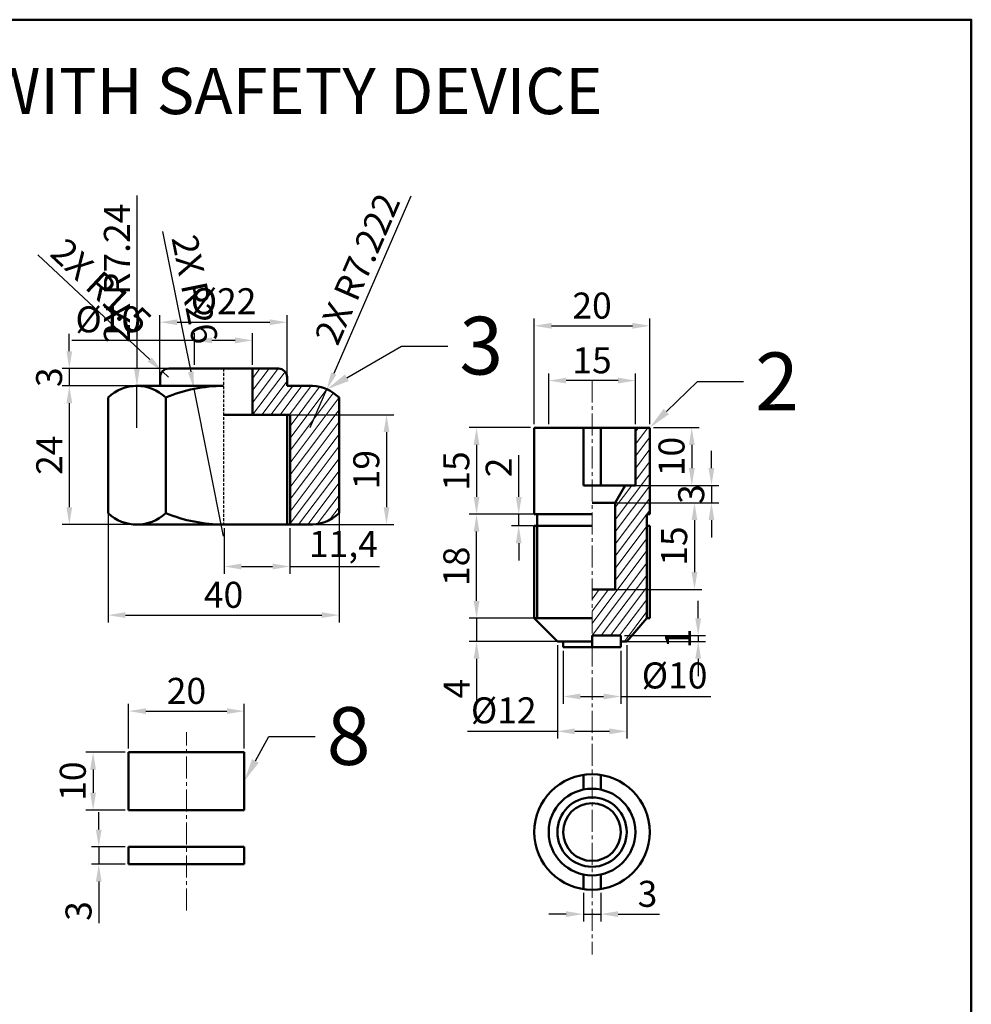
# Model space of a CAD drawing. Units: millimetres. Extents: x 418 to 773, y -46 to 294.
# Tile 7 of 7: x 609 to 773, y 124 to 294. Entities that reach past the tile are written whole.
import ezdxf
from ezdxf import colors
from ezdxf.entities.mleader import LeaderData, LeaderLine
from ezdxf.math import Vec2, Vec3

# ---------------------------------------------------------------- set-up
doc = ezdxf.new("R2010")
doc.units = ezdxf.units.MM
doc.header["$LTSCALE"] = 0.2
doc.linetypes.add('CENTER2', pattern=[28.575, 19.05, -3.175, 3.175, -3.175])
doc.linetypes.add('DASHED', pattern=[19.05, 12.7, -6.35])
for name, color, linetype, lineweight in [('M-CNTR', 1, 'CENTER2', 18), ('M-DIMS', 2, 'Continuous', 25), ('M-HATC', 8, 'Continuous', 18), ('M-HIDN', 4, 'DASHED', 25), ('M-OUTL', 7, 'Continuous', 50), ('M-TEXT', 3, 'Continuous', 25), ('M-TTLB', 7, 'Continuous', 50)]:
    doc.layers.add(name, color=color, linetype=linetype, lineweight=lineweight)
doc.styles.get("Standard").update_dxf_attribs({"font": 'arial.ttf'})
doc.dimstyles.new('ISO-25', dxfattribs={"dimtxt": 4.5, "dimasz": 3, "dimexe": 1.25, "dimexo": 0.625, "dimtad": 1, "dimdec": 1, "dimtxsty": 'Standard', "dimcen": 2.5, "dimadec": 0, "dimazin": 0, "dimtfac": 1, "dimtdec": 1, "dimtmove": 0, "dimatfit": 3, "dimfxl": 1, "dimarcsym": 0})

# ---------------------------------------------------------------- blocks, each defined once
blk = doc.blocks.new('*D43')
at = {"layer": 'Defpoints', "color": 0, "ltscale": 0.2, "transparency": 16777216}
for p in [(643.92, 207.02), (655.34, 207.02), (655.34, 199.76)]:
    blk.add_point(p, dxfattribs=at)
at = {"layer": 'M-DIMS', "color": 0, "lineweight": -2, "ltscale": 0.2, "transparency": 16777216}
for p, q in [((643.92, 206.39), (643.92, 198.51)), ((655.34, 206.39), (655.34, 198.51)), ((646.92, 199.76), (652.34, 199.76)), ((655.34, 199.76), (670.84, 199.76))]:
    blk.add_line(p, q, dxfattribs=at)
at = {"layer": 'M-DIMS', "color": 0, "ltscale": 0.2, "transparency": 16777216}
for points in [[(646.92, 200.26), (646.92, 199.26), (643.92, 199.76)], [(652.34, 200.26), (652.34, 199.26), (655.34, 199.76)]]:
    blk.add_solid(points, dxfattribs=at)
at = {"layer": 'M-DIMS', "color": 0, "ltscale": 0.2, "transparency": 16777216, "insert": (664.59, 203.09), "char_height": 4.5, "attachment_point": 5}
blk.add_mtext('11,4', dxfattribs=at)
blk = doc.blocks.new('*D44')
at = {"layer": 'Defpoints', "color": 0, "ltscale": 0.2, "transparency": 16777216}
for p in [(623.84, 214.93), (663.84, 214.93), (663.84, 191.34)]:
    blk.add_point(p, dxfattribs=at)
at = {"layer": 'M-DIMS', "color": 0, "lineweight": -2, "ltscale": 0.2, "transparency": 16777216}
for p, q in [((623.84, 214.31), (623.84, 190.09)), ((663.84, 214.31), (663.84, 190.09)), ((626.84, 191.34), (660.84, 191.34))]:
    blk.add_line(p, q, dxfattribs=at)
at = {"layer": 'M-DIMS', "color": 0, "ltscale": 0.2, "transparency": 16777216}
for points in [[(626.84, 191.84), (626.84, 190.84), (623.84, 191.34)], [(660.84, 191.84), (660.84, 190.84), (663.84, 191.34)]]:
    blk.add_solid(points, dxfattribs=at)
at = {"layer": 'M-DIMS', "color": 0, "ltscale": 0.2, "transparency": 16777216, "insert": (643.84, 194.27), "char_height": 4.5, "attachment_point": 5}
blk.add_mtext('40', dxfattribs=at)
blk = doc.blocks.new('*D45')
at = {"layer": 'Defpoints', "color": 0, "ltscale": 0.2, "transparency": 16777216}
for p in [(654.84, 226.02), (654.84, 207.02), (672.05, 207.02)]:
    blk.add_point(p, dxfattribs=at)
at = {"layer": 'M-DIMS', "color": 0, "lineweight": -2, "ltscale": 0.2, "transparency": 16777216}
for p, q in [((655.47, 226.02), (673.3, 226.02)), ((672.05, 223.02), (672.05, 210.02)), ((655.47, 207.02), (673.3, 207.02))]:
    blk.add_line(p, q, dxfattribs=at)
at = {"layer": 'M-DIMS', "color": 0, "ltscale": 0.2, "transparency": 16777216}
for points in [[(671.55, 223.02), (672.55, 223.02), (672.05, 226.02)], [(671.55, 210.02), (672.55, 210.02), (672.05, 207.02)]]:
    blk.add_solid(points, dxfattribs=at)
at = {"layer": 'M-DIMS', "color": 0, "ltscale": 0.2, "transparency": 16777216, "insert": (669.13, 216.52), "char_height": 4.5, "attachment_point": 5, "rotation": 90}
blk.add_mtext('19', dxfattribs=at)
blk = doc.blocks.new('*D46')
at = {"layer": 'Defpoints', "color": 0, "ltscale": 0.2, "transparency": 16777216}
for p in [(632.84, 231.02), (617.14, 207.02), (632.84, 207.02)]:
    blk.add_point(p, dxfattribs=at)
at = {"layer": 'M-DIMS', "color": 0, "lineweight": -2, "ltscale": 0.2, "transparency": 16777216}
for p, q in [((632.22, 231.02), (615.89, 231.02)), ((617.14, 228.02), (617.14, 210.02)), ((632.22, 207.02), (615.89, 207.02))]:
    blk.add_line(p, q, dxfattribs=at)
at = {"layer": 'M-DIMS', "color": 0, "ltscale": 0.2, "transparency": 16777216}
for points in [[(616.64, 228.02), (617.64, 228.02), (617.14, 231.02)], [(616.64, 210.02), (617.64, 210.02), (617.14, 207.02)]]:
    blk.add_solid(points, dxfattribs=at)
at = {"layer": 'M-DIMS', "color": 0, "ltscale": 0.2, "transparency": 16777216, "insert": (614.26, 219.02), "char_height": 4.5, "attachment_point": 5, "rotation": 90}
blk.add_mtext('24', dxfattribs=at)
blk = doc.blocks.new('*D47')
at = {"layer": 'Defpoints', "color": 0, "ltscale": 0.2, "transparency": 16777216}
for p in [(642.2, 234.02), (617.14, 231.02), (642.2, 231.02)]:
    blk.add_point(p, dxfattribs=at)
at = {"layer": 'M-DIMS', "color": 0, "lineweight": -2, "ltscale": 0.2, "transparency": 16777216}
for p, q in [((617.14, 237.02), (617.14, 240.02)), ((641.58, 234.02), (615.89, 234.02)), ((617.14, 234.02), (617.14, 231.02)), ((641.58, 231.02), (615.89, 231.02)), ((617.14, 228.02), (617.14, 225.02))]:
    blk.add_line(p, q, dxfattribs=at)
at = {"layer": 'M-DIMS', "color": 0, "ltscale": 0.2, "transparency": 16777216}
for points in [[(616.64, 237.02), (617.64, 237.02), (617.14, 234.02)], [(616.64, 228.02), (617.64, 228.02), (617.14, 231.02)]]:
    blk.add_solid(points, dxfattribs=at)
at = {"layer": 'M-DIMS', "color": 0, "ltscale": 0.2, "transparency": 16777216, "insert": (614.22, 232.52), "char_height": 4.5, "attachment_point": 5, "rotation": 90}
blk.add_mtext('3', dxfattribs=at)
blk = doc.blocks.new('*D48')
at = {"layer": 'Defpoints', "color": 0, "ltscale": 0.2, "transparency": 16777216}
for p in [(654.84, 242.04), (632.84, 231.02), (654.84, 231.02)]:
    blk.add_point(p, dxfattribs=at)
at = {"layer": 'M-DIMS', "color": 0, "lineweight": -2, "ltscale": 0.2, "transparency": 16777216}
for p, q in [((632.84, 231.64), (632.84, 243.29)), ((635.84, 242.04), (651.84, 242.04)), ((654.84, 231.64), (654.84, 243.29))]:
    blk.add_line(p, q, dxfattribs=at)
at = {"layer": 'M-DIMS', "color": 0, "ltscale": 0.2, "transparency": 16777216}
for points in [[(635.84, 242.54), (635.84, 241.54), (632.84, 242.04)], [(651.84, 242.54), (651.84, 241.54), (654.84, 242.04)]]:
    blk.add_solid(points, dxfattribs=at)
at = {"layer": 'M-DIMS', "color": 0, "ltscale": 0.2, "transparency": 16777216, "insert": (643.84, 245.09), "char_height": 4.5, "attachment_point": 5}
blk.add_mtext('%%C22', dxfattribs=at)
blk = doc.blocks.new('*D49')
at = {"layer": 'Defpoints', "color": 0, "ltscale": 0.2, "transparency": 16777216}
for p in [(638.84, 238.9), (638.84, 234.02), (648.84, 234.02)]:
    blk.add_point(p, dxfattribs=at)
at = {"layer": 'M-DIMS', "color": 0, "lineweight": -2, "ltscale": 0.2, "transparency": 16777216}
for p, q in [((638.84, 238.9), (617.6, 238.9)), ((638.84, 234.64), (638.84, 240.15)), ((645.84, 238.9), (641.84, 238.9)), ((648.84, 234.64), (648.84, 240.15))]:
    blk.add_line(p, q, dxfattribs=at)
at = {"layer": 'M-DIMS', "color": 0, "ltscale": 0.2, "transparency": 16777216}
for points in [[(641.84, 239.4), (641.84, 238.4), (638.84, 238.9)], [(645.84, 239.4), (645.84, 238.4), (648.84, 238.9)]]:
    blk.add_solid(points, dxfattribs=at)
at = {"layer": 'M-DIMS', "color": 0, "ltscale": 0.2, "transparency": 16777216, "insert": (623.89, 241.95), "char_height": 4.5, "attachment_point": 5}
blk.add_mtext('%%C10', dxfattribs=at)
blk = doc.blocks.new('*U50')
at = {"layer": 'M-CNTR', "color": 0, "transparency": 16777216}
blk.add_line((0, -22.42), (0, 8.5), dxfattribs=at)
blk = doc.blocks.new('*D51')
at = {"layer": 'Defpoints', "color": 0, "ltscale": 0.2, "transparency": 16777216}
for p in [(647.41, 174.72), (627.41, 167.6), (647.41, 167.6)]:
    blk.add_point(p, dxfattribs=at)
at = {"layer": 'M-DIMS', "color": 0, "lineweight": -2, "ltscale": 0.2, "transparency": 16777216}
for p, q in [((627.41, 168.23), (627.41, 175.97)), ((647.41, 168.23), (647.41, 175.97)), ((630.41, 174.72), (644.41, 174.72))]:
    blk.add_line(p, q, dxfattribs=at)
at = {"layer": 'M-DIMS', "color": 0, "ltscale": 0.2, "transparency": 16777216}
for points in [[(630.41, 175.22), (630.41, 174.22), (627.41, 174.72)], [(644.41, 175.22), (644.41, 174.22), (647.41, 174.72)]]:
    blk.add_solid(points, dxfattribs=at)
at = {"layer": 'M-DIMS', "color": 0, "ltscale": 0.2, "transparency": 16777216, "insert": (637.41, 177.64), "char_height": 4.5, "attachment_point": 5}
blk.add_mtext('20', dxfattribs=at)
blk = doc.blocks.new('*D52')
at = {"layer": 'Defpoints', "color": 0, "ltscale": 0.2, "transparency": 16777216}
for p in [(627.41, 167.6), (621.26, 157.6), (627.41, 157.6)]:
    blk.add_point(p, dxfattribs=at)
at = {"layer": 'M-DIMS', "color": 0, "lineweight": -2, "ltscale": 0.2, "transparency": 16777216}
for p, q in [((626.79, 167.6), (620.01, 167.6)), ((621.26, 164.6), (621.26, 160.6)), ((626.79, 157.6), (620.01, 157.6))]:
    blk.add_line(p, q, dxfattribs=at)
at = {"layer": 'M-DIMS', "color": 0, "ltscale": 0.2, "transparency": 16777216}
for points in [[(620.76, 164.6), (621.76, 164.6), (621.26, 167.6)], [(620.76, 160.6), (621.76, 160.6), (621.26, 157.6)]]:
    blk.add_solid(points, dxfattribs=at)
at = {"layer": 'M-DIMS', "color": 0, "ltscale": 0.2, "transparency": 16777216, "insert": (618.33, 162.6), "char_height": 4.5, "attachment_point": 5, "rotation": 90}
blk.add_mtext('10', dxfattribs=at)
blk = doc.blocks.new('*D53')
at = {"layer": 'Defpoints', "color": 0, "ltscale": 0.2, "transparency": 16777216}
for p in [(627.41, 151.22), (622.24, 148.22), (627.41, 148.22)]:
    blk.add_point(p, dxfattribs=at)
at = {"layer": 'M-DIMS', "color": 0, "lineweight": -2, "ltscale": 0.2, "transparency": 16777216}
for p, q in [((622.24, 154.22), (622.24, 157.22)), ((626.79, 151.22), (620.99, 151.22)), ((622.24, 151.22), (622.24, 148.22)), ((626.79, 148.22), (620.99, 148.22)), ((622.24, 145.22), (622.24, 138.03))]:
    blk.add_line(p, q, dxfattribs=at)
at = {"layer": 'M-DIMS', "color": 0, "ltscale": 0.2, "transparency": 16777216}
for points in [[(621.74, 154.22), (622.74, 154.22), (622.24, 151.22)], [(621.74, 145.22), (622.74, 145.22), (622.24, 148.22)]]:
    blk.add_solid(points, dxfattribs=at)
at = {"layer": 'M-DIMS', "color": 0, "ltscale": 0.2, "transparency": 16777216, "insert": (619.32, 140.12), "char_height": 4.5, "attachment_point": 5, "rotation": 90}
blk.add_mtext('3', dxfattribs=at)
blk = doc.blocks.new('*U54')
at = {"layer": 'M-CNTR', "color": 0, "transparency": 16777216}
blk.add_line((0, 24.41), (0, -74.97), dxfattribs=at)
blk = doc.blocks.new('*D55')
at = {"layer": 'Defpoints', "color": 0, "ltscale": 0.2, "transparency": 16777216}
for p in [(717.62, 241.42), (697.62, 223.79), (717.62, 223.79)]:
    blk.add_point(p, dxfattribs=at)
at = {"layer": 'M-DIMS', "color": 0, "lineweight": -2, "ltscale": 0.2, "transparency": 16777216}
for p, q in [((697.62, 224.41), (697.62, 242.67)), ((717.62, 224.41), (717.62, 242.67)), ((700.62, 241.42), (714.62, 241.42))]:
    blk.add_line(p, q, dxfattribs=at)
at = {"layer": 'M-DIMS', "color": 0, "ltscale": 0.2, "transparency": 16777216}
for points in [[(700.62, 241.92), (700.62, 240.92), (697.62, 241.42)], [(714.62, 241.92), (714.62, 240.92), (717.62, 241.42)]]:
    blk.add_solid(points, dxfattribs=at)
at = {"layer": 'M-DIMS', "color": 0, "ltscale": 0.2, "transparency": 16777216, "insert": (707.62, 244.34), "char_height": 4.5, "attachment_point": 5}
blk.add_mtext('20', dxfattribs=at)
blk = doc.blocks.new('*D56')
at = {"layer": 'Defpoints', "color": 0, "ltscale": 0.2, "transparency": 16777216}
for p in [(700.12, 231.94), (700.12, 223.79), (715.12, 223.79)]:
    blk.add_point(p, dxfattribs=at)
at = {"layer": 'M-DIMS', "color": 0, "lineweight": -2, "ltscale": 0.2, "transparency": 16777216}
for p, q in [((700.12, 224.41), (700.12, 233.19)), ((712.12, 231.94), (703.12, 231.94)), ((715.12, 224.41), (715.12, 233.19))]:
    blk.add_line(p, q, dxfattribs=at)
at = {"layer": 'M-DIMS', "color": 0, "ltscale": 0.2, "transparency": 16777216}
for points in [[(703.12, 232.44), (703.12, 231.44), (700.12, 231.94)], [(712.12, 232.44), (712.12, 231.44), (715.12, 231.94)]]:
    blk.add_solid(points, dxfattribs=at)
at = {"layer": 'M-DIMS', "color": 0, "ltscale": 0.2, "transparency": 16777216, "insert": (707.62, 234.87), "char_height": 4.5, "attachment_point": 5}
blk.add_mtext('15', dxfattribs=at)
blk = doc.blocks.new('*D57')
at = {"layer": 'Defpoints', "color": 0, "ltscale": 0.2, "transparency": 16777216}
for p in [(697.62, 223.79), (687.63, 208.79), (697.62, 208.79)]:
    blk.add_point(p, dxfattribs=at)
at = {"layer": 'M-DIMS', "color": 0, "lineweight": -2, "ltscale": 0.2, "transparency": 16777216}
for p, q in [((696.99, 223.79), (686.38, 223.79)), ((687.63, 220.79), (687.63, 211.79)), ((696.99, 208.79), (686.38, 208.79))]:
    blk.add_line(p, q, dxfattribs=at)
at = {"layer": 'M-DIMS', "color": 0, "ltscale": 0.2, "transparency": 16777216}
for points in [[(687.13, 220.79), (688.13, 220.79), (687.63, 223.79)], [(687.13, 211.79), (688.13, 211.79), (687.63, 208.79)]]:
    blk.add_solid(points, dxfattribs=at)
at = {"layer": 'M-DIMS', "color": 0, "ltscale": 0.2, "transparency": 16777216, "insert": (684.71, 216.29), "char_height": 4.5, "attachment_point": 5, "rotation": 90}
blk.add_mtext('15', dxfattribs=at)
blk = doc.blocks.new('*D58')
at = {"layer": 'Defpoints', "color": 0, "ltscale": 0.2, "transparency": 16777216}
for p in [(698.12, 208.79), (694.93, 206.79), (698.12, 206.79)]:
    blk.add_point(p, dxfattribs=at)
at = {"layer": 'M-DIMS', "color": 0, "lineweight": -2, "ltscale": 0.2, "transparency": 16777216}
for p, q in [((694.93, 211.79), (694.93, 219.02)), ((697.49, 208.79), (693.68, 208.79)), ((694.93, 206.79), (694.93, 208.79)), ((697.49, 206.79), (693.68, 206.79)), ((694.93, 203.79), (694.93, 200.79))]:
    blk.add_line(p, q, dxfattribs=at)
at = {"layer": 'M-DIMS', "color": 0, "ltscale": 0.2, "transparency": 16777216}
for points in [[(694.43, 211.79), (695.43, 211.79), (694.93, 208.79)], [(694.43, 203.79), (695.43, 203.79), (694.93, 206.79)]]:
    blk.add_solid(points, dxfattribs=at)
at = {"layer": 'M-DIMS', "color": 0, "ltscale": 0.2, "transparency": 16777216, "insert": (692.05, 216.9), "char_height": 4.5, "attachment_point": 5, "rotation": 90}
blk.add_mtext('2', dxfattribs=at)
blk = doc.blocks.new('*D59')
at = {"layer": 'Defpoints', "color": 0, "ltscale": 0.2, "transparency": 16777216}
for p in [(687.63, 208.79), (700.91, 208.79), (700.91, 190.79)]:
    blk.add_point(p, dxfattribs=at)
at = {"layer": 'M-DIMS', "color": 0, "lineweight": -2, "ltscale": 0.2, "transparency": 16777216}
for p, q in [((700.29, 208.79), (686.38, 208.79)), ((687.63, 193.79), (687.63, 205.79)), ((700.29, 190.79), (686.38, 190.79))]:
    blk.add_line(p, q, dxfattribs=at)
at = {"layer": 'M-DIMS', "color": 0, "ltscale": 0.2, "transparency": 16777216}
for points in [[(687.13, 205.79), (688.13, 205.79), (687.63, 208.79)], [(687.13, 193.79), (688.13, 193.79), (687.63, 190.79)]]:
    blk.add_solid(points, dxfattribs=at)
at = {"layer": 'M-DIMS', "color": 0, "ltscale": 0.2, "transparency": 16777216, "insert": (684.71, 199.79), "char_height": 4.5, "attachment_point": 5, "rotation": 90}
blk.add_mtext('18', dxfattribs=at)
blk = doc.blocks.new('*D60')
at = {"layer": 'Defpoints', "color": 0, "ltscale": 0.2, "transparency": 16777216}
for p in [(702.62, 190.79), (687.63, 186.79), (702.62, 186.79)]:
    blk.add_point(p, dxfattribs=at)
at = {"layer": 'M-DIMS', "color": 0, "lineweight": -2, "ltscale": 0.2, "transparency": 16777216}
for p, q in [((687.63, 193.79), (687.63, 196.79)), ((701.99, 190.79), (686.38, 190.79)), ((687.63, 190.79), (687.63, 186.79)), ((701.99, 186.79), (686.38, 186.79)), ((687.63, 183.79), (687.63, 176.43))]:
    blk.add_line(p, q, dxfattribs=at)
at = {"layer": 'M-DIMS', "color": 0, "ltscale": 0.2, "transparency": 16777216}
for points in [[(687.13, 193.79), (688.13, 193.79), (687.63, 190.79)], [(687.13, 183.79), (688.13, 183.79), (687.63, 186.79)]]:
    blk.add_solid(points, dxfattribs=at)
at = {"layer": 'M-DIMS', "color": 0, "ltscale": 0.2, "transparency": 16777216, "insert": (684.76, 178.61), "char_height": 4.5, "attachment_point": 5, "rotation": 90}
blk.add_mtext('4', dxfattribs=at)
blk = doc.blocks.new('*D61')
at = {"layer": 'Defpoints', "color": 0, "ltscale": 0.2, "transparency": 16777216}
for p in [(702.62, 185.79), (712.62, 185.79), (712.62, 177.26)]:
    blk.add_point(p, dxfattribs=at)
at = {"layer": 'M-DIMS', "color": 0, "lineweight": -2, "ltscale": 0.2, "transparency": 16777216}
for p, q in [((702.62, 185.16), (702.62, 176.01)), ((712.62, 185.16), (712.62, 176.01)), ((705.62, 177.26), (709.62, 177.26)), ((712.62, 177.26), (728.19, 177.26))]:
    blk.add_line(p, q, dxfattribs=at)
at = {"layer": 'M-DIMS', "color": 0, "ltscale": 0.2, "transparency": 16777216}
for points in [[(705.62, 177.76), (705.62, 176.76), (702.62, 177.26)], [(709.62, 177.76), (709.62, 176.76), (712.62, 177.26)]]:
    blk.add_solid(points, dxfattribs=at)
at = {"layer": 'M-DIMS', "color": 0, "ltscale": 0.2, "transparency": 16777216, "insert": (721.91, 180.31), "char_height": 4.5, "attachment_point": 5}
blk.add_mtext('%%C10', dxfattribs=at)
blk = doc.blocks.new('*D62')
at = {"layer": 'Defpoints', "color": 0, "ltscale": 0.2, "transparency": 16777216}
for p in [(701.62, 186.79), (713.62, 186.79), (713.62, 171.22)]:
    blk.add_point(p, dxfattribs=at)
at = {"layer": 'M-DIMS', "color": 0, "lineweight": -2, "ltscale": 0.2, "transparency": 16777216}
for p, q in [((701.62, 186.16), (701.62, 169.97)), ((713.62, 186.16), (713.62, 169.97)), ((701.62, 171.22), (686.07, 171.22)), ((710.62, 171.22), (704.62, 171.22))]:
    blk.add_line(p, q, dxfattribs=at)
at = {"layer": 'M-DIMS', "color": 0, "ltscale": 0.2, "transparency": 16777216}
for points in [[(704.62, 171.72), (704.62, 170.72), (701.62, 171.22)], [(710.62, 171.72), (710.62, 170.72), (713.62, 171.22)]]:
    blk.add_solid(points, dxfattribs=at)
at = {"layer": 'M-DIMS', "color": 0, "ltscale": 0.2, "transparency": 16777216, "insert": (692.34, 174.27), "char_height": 4.5, "attachment_point": 5}
blk.add_mtext('%%C12', dxfattribs=at)
blk = doc.blocks.new('*D63')
at = {"layer": 'Defpoints', "color": 0, "ltscale": 0.2, "transparency": 16777216}
for p in [(717.62, 223.79), (715.12, 213.79), (724.89, 213.79)]:
    blk.add_point(p, dxfattribs=at)
at = {"layer": 'M-DIMS', "color": 0, "lineweight": -2, "ltscale": 0.2, "transparency": 16777216}
for p, q in [((718.24, 223.79), (726.14, 223.79)), ((724.89, 220.79), (724.89, 216.79)), ((715.74, 213.79), (726.14, 213.79))]:
    blk.add_line(p, q, dxfattribs=at)
at = {"layer": 'M-DIMS', "color": 0, "ltscale": 0.2, "transparency": 16777216}
for points in [[(724.39, 220.79), (725.39, 220.79), (724.89, 223.79)], [(724.39, 216.79), (725.39, 216.79), (724.89, 213.79)]]:
    blk.add_solid(points, dxfattribs=at)
at = {"layer": 'M-DIMS', "color": 0, "ltscale": 0.2, "transparency": 16777216, "insert": (721.96, 218.79), "char_height": 4.5, "attachment_point": 5, "rotation": 90}
blk.add_mtext('10', dxfattribs=at)
blk = doc.blocks.new('*D64')
at = {"layer": 'Defpoints', "color": 0, "ltscale": 0.2, "transparency": 16777216}
for p in [(712.12, 213.79), (711.62, 210.79), (728.29, 210.79)]:
    blk.add_point(p, dxfattribs=at)
at = {"layer": 'M-DIMS', "color": 0, "lineweight": -2, "ltscale": 0.2, "transparency": 16777216}
for p, q in [((728.29, 216.79), (728.29, 219.79)), ((712.74, 213.79), (729.54, 213.79)), ((728.29, 213.79), (728.29, 210.79)), ((712.24, 210.79), (729.54, 210.79)), ((728.29, 207.79), (728.29, 204.79))]:
    blk.add_line(p, q, dxfattribs=at)
at = {"layer": 'M-DIMS', "color": 0, "ltscale": 0.2, "transparency": 16777216}
for points in [[(727.79, 216.79), (728.79, 216.79), (728.29, 213.79)], [(727.79, 207.79), (728.79, 207.79), (728.29, 210.79)]]:
    blk.add_solid(points, dxfattribs=at)
at = {"layer": 'M-DIMS', "color": 0, "ltscale": 0.2, "transparency": 16777216, "insert": (725.37, 212.29), "char_height": 4.5, "attachment_point": 5, "rotation": 90}
blk.add_mtext('3', dxfattribs=at)
blk = doc.blocks.new('*D65')
at = {"layer": 'Defpoints', "color": 0, "ltscale": 0.2, "transparency": 16777216}
for p in [(709.62, 210.79), (709.62, 195.79), (725.35, 195.79)]:
    blk.add_point(p, dxfattribs=at)
at = {"layer": 'M-DIMS', "color": 0, "lineweight": -2, "ltscale": 0.2, "transparency": 16777216}
for p, q in [((710.24, 210.79), (726.6, 210.79)), ((725.35, 207.79), (725.35, 198.79)), ((710.24, 195.79), (726.6, 195.79))]:
    blk.add_line(p, q, dxfattribs=at)
at = {"layer": 'M-DIMS', "color": 0, "ltscale": 0.2, "transparency": 16777216}
for points in [[(724.85, 207.79), (725.85, 207.79), (725.35, 210.79)], [(724.85, 198.79), (725.85, 198.79), (725.35, 195.79)]]:
    blk.add_solid(points, dxfattribs=at)
at = {"layer": 'M-DIMS', "color": 0, "ltscale": 0.2, "transparency": 16777216, "insert": (722.42, 203.29), "char_height": 4.5, "attachment_point": 5, "rotation": 90}
blk.add_mtext('15', dxfattribs=at)
blk = doc.blocks.new('*D66')
at = {"layer": 'Defpoints', "color": 0, "ltscale": 0.2, "transparency": 16777216}
for p in [(712.62, 187.79), (712.62, 186.79), (725.99, 186.79)]:
    blk.add_point(p, dxfattribs=at)
at = {"layer": 'M-DIMS', "color": 0, "lineweight": -2, "ltscale": 0.2, "transparency": 16777216}
for p, q in [((725.99, 190.79), (725.99, 193.79)), ((713.24, 187.79), (727.24, 187.79)), ((725.99, 187.79), (725.99, 186.79)), ((713.24, 186.79), (727.24, 186.79)), ((725.99, 183.79), (725.99, 180.79))]:
    blk.add_line(p, q, dxfattribs=at)
at = {"layer": 'M-DIMS', "color": 0, "ltscale": 0.2, "transparency": 16777216}
for points in [[(725.49, 190.79), (726.49, 190.79), (725.99, 187.79)], [(725.49, 183.79), (726.49, 183.79), (725.99, 186.79)]]:
    blk.add_solid(points, dxfattribs=at)
at = {"layer": 'M-DIMS', "color": 0, "ltscale": 0.2, "transparency": 16777216, "insert": (723.11, 187.29), "char_height": 4.5, "attachment_point": 5, "rotation": 90}
blk.add_mtext('1', dxfattribs=at)
blk = doc.blocks.new('*D67')
at = {"layer": 'Defpoints', "color": 0, "ltscale": 0.2, "transparency": 16777216}
for p in [(706.12, 143.9), (709.12, 143.9), (709.12, 139.58)]:
    blk.add_point(p, dxfattribs=at)
at = {"layer": 'M-DIMS', "color": 0, "lineweight": -2, "ltscale": 0.2, "transparency": 16777216}
for p, q in [((706.12, 143.28), (706.12, 138.33)), ((709.12, 143.28), (709.12, 138.33)), ((703.12, 139.58), (700.12, 139.58)), ((706.12, 139.58), (709.12, 139.58)), ((712.12, 139.58), (719.31, 139.58))]:
    blk.add_line(p, q, dxfattribs=at)
at = {"layer": 'M-DIMS', "color": 0, "ltscale": 0.2, "transparency": 16777216}
for points in [[(703.12, 140.08), (703.12, 139.08), (706.12, 139.58)], [(712.12, 140.08), (712.12, 139.08), (709.12, 139.58)]]:
    blk.add_solid(points, dxfattribs=at)
at = {"layer": 'M-DIMS', "color": 0, "ltscale": 0.2, "transparency": 16777216, "insert": (717.22, 142.51), "char_height": 4.5, "attachment_point": 5}
blk.add_mtext('3', dxfattribs=at)
blk = doc.blocks.new('*D106')
at = {"layer": 'Defpoints', "color": 0, "ltscale": 0.2, "transparency": 16777216}
for p in [(638.74, 230.51), (643.84, 205.02)]:
    blk.add_point(p, dxfattribs=at)
at = {"layer": 'M-DIMS', "color": 0, "lineweight": -2, "ltscale": 0.2, "transparency": 16777216}
for p, q in [((633.3, 257.72), (638.16, 233.45)), ((643.84, 205.02), (638.74, 230.51))]:
    blk.add_line(p, q, dxfattribs=at)
at = {"layer": 'M-DIMS', "color": 0, "ltscale": 0.2, "transparency": 16777216}
blk.add_solid([(638.65, 233.55), (637.67, 233.36), (638.74, 230.51)], dxfattribs=at)
at = {"layer": 'M-DIMS', "color": 0, "ltscale": 0.2, "transparency": 16777216, "insert": (638.3, 247.63), "char_height": 4.5, "attachment_point": 5, "rotation": 281.3094}
blk.add_mtext('2X R26', dxfattribs=at)
blk = doc.blocks.new('*D107')
at = {"layer": 'Defpoints', "color": 0, "ltscale": 0.2, "transparency": 16777216}
for p in [(628.84, 231.02), (628.84, 223.78)]:
    blk.add_point(p, dxfattribs=at)
at = {"layer": 'M-DIMS', "color": 0, "lineweight": -2, "ltscale": 0.2, "transparency": 16777216}
for p, q in [((628.84, 263.99), (628.84, 234.02)), ((628.84, 223.78), (628.84, 231.02))]:
    blk.add_line(p, q, dxfattribs=at)
at = {"layer": 'M-DIMS', "color": 0, "ltscale": 0.2, "transparency": 16777216}
blk.add_solid([(628.34, 234.02), (629.34, 234.02), (628.84, 231.02)], dxfattribs=at)
at = {"layer": 'M-DIMS', "color": 0, "ltscale": 0.2, "transparency": 16777216, "insert": (625.96, 250.51), "char_height": 4.5, "attachment_point": 5, "rotation": 89.9988}
blk.add_mtext('2X R7.24', dxfattribs=at)
blk = doc.blocks.new('*D108')
at = {"layer": 'Defpoints', "color": 0, "ltscale": 0.2, "transparency": 16777216}
for p in [(661.72, 230.43), (658.84, 223.81)]:
    blk.add_point(p, dxfattribs=at)
at = {"layer": 'M-DIMS', "color": 0, "lineweight": -2, "ltscale": 0.2, "transparency": 16777216}
for p, q in [((676.24, 263.85), (662.92, 233.18)), ((658.84, 223.81), (661.72, 230.43))]:
    blk.add_line(p, q, dxfattribs=at)
at = {"layer": 'M-DIMS', "color": 0, "ltscale": 0.2, "transparency": 16777216}
blk.add_solid([(662.46, 233.38), (663.37, 232.98), (661.72, 230.43)], dxfattribs=at)
at = {"layer": 'M-DIMS', "color": 0, "ltscale": 0.2, "transparency": 16777216, "insert": (667.53, 251.04), "char_height": 4.5, "attachment_point": 5, "rotation": 66.5204}
blk.add_mtext('2X R7.222', dxfattribs=at)
blk = doc.blocks.new('*D109')
at = {"layer": 'Defpoints', "color": 0, "ltscale": 0.2, "transparency": 16777216}
for p in [(633.25, 233.54), (634.34, 232.52)]:
    blk.add_point(p, dxfattribs=at)
at = {"layer": 'M-DIMS', "color": 0, "lineweight": -2, "ltscale": 0.2, "transparency": 16777216}
for p, q in [((611.69, 253.72), (631.06, 235.59)), ((634.34, 232.52), (633.25, 233.54))]:
    blk.add_line(p, q, dxfattribs=at)
at = {"layer": 'M-DIMS', "color": 0, "ltscale": 0.2, "transparency": 16777216}
blk.add_solid([(631.4, 235.96), (630.72, 235.23), (633.25, 233.54)], dxfattribs=at)
at = {"layer": 'M-DIMS', "color": 0, "ltscale": 0.2, "transparency": 16777216, "insert": (622.28, 247.82), "char_height": 4.5, "attachment_point": 5, "rotation": 316.8922}
blk.add_mtext('2X R1.5', dxfattribs=at)

msp = doc.modelspace()

# ---------------------------------------------------------------- hatches: boundary and pattern name
at = {"layer": 'M-HATC', "ltscale": 0.2}
h = msp.add_hatch(dxfattribs=at)
h.set_pattern_fill('ANSI31', color=256, scale=0.4, angle=8)
h.set_pattern_definition([(53, (-50.2854, 17.8154), (-1.014267, 0.764305), [])])
h.paths.add_polyline_path([(663.8429, 229.0175, 0.17937471), (659.2384, 231.0175), (654.8429, 231.0175), (654.8429, 232.5175, 0.41421356), (653.3429, 234.0175), (648.8429, 234.0175), (648.8429, 226.0175), (655.3429, 226.0175), (655.3429, 207.0175), (659.2384, 207.0175, 0.17937471), (663.8429, 209.0175)])
h = msp.add_hatch(dxfattribs=at)
h.set_pattern_fill('ANSI31', color=256, scale=0.4, angle=8)
h.set_pattern_definition([(53, (-17.2468, 29.8724), (-1.014267, 0.764305), [])])
h.paths.add_polyline_path([(717.1175, 206.7888), (711.6175, 206.7888), (711.6175, 195.7888), (707.6175, 195.7888), (707.6175, 187.7888), (712.6175, 187.7888), (712.6175, 186.7888), (713.6175, 186.7888), (717.1175, 190.7888)])
h.paths.add_polyline_path([(717.6175, 223.7888), (715.1175, 223.7888), (715.1175, 213.7888), (713.3496, 213.7888), (711.6175, 210.7888), (711.6175, 206.7888), (717.1175, 206.7888), (717.1175, 208.7888), (717.6175, 208.7888)])

# ---------------------------------------------------------------- linework, layer by layer
at = {"layer": 'M-HIDN', "ltscale": 0.2}
msp.add_line((643.8429, 234.0175), (643.8429, 207.0175), dxfattribs=at)
at = {"layer": 'M-OUTL', "ltscale": 0.2}
for p, q in [((653.3429, 234.0175), (634.3429, 234.0175)), ((648.8429, 234.0175), (648.8429, 226.0175)), ((632.8429, 232.5175), (632.8429, 231.0175)), ((654.8429, 231.0175), (654.8429, 232.5175)), ((654.8429, 232.5175), (654.8429, 231.0175)), ((643.8429, 231.0175), (628.6077, 231.0175)), ((659.2384, 231.0175), (654.8429, 231.0175)), ((623.8429, 229.0175), (623.8429, 209.0175)), ((633.8429, 229.0175), (633.8429, 209.0175)), ((663.8429, 209.0175), (663.8429, 229.0175)), ((643.8429, 226.0175), (655.3429, 226.0175)), ((654.8429, 226.0175), (654.8429, 207.0175)), ((655.3429, 226.0175), (655.3429, 207.0175)), ((697.6175, 223.7888), (717.6175, 223.7888)), ((697.6175, 223.7888), (697.6175, 208.7888)), ((706.1175, 213.7888), (706.1175, 223.7888)), ((707.6175, 223.7888), (709.1175, 223.7888)), ((707.6175, 223.7888), (715.1175, 223.7888)), ((709.1175, 223.7888), (709.1175, 213.7888)), ((715.1175, 223.7888), (715.1175, 213.7888)), ((717.6175, 208.7888), (717.6175, 223.7888)), ((709.1175, 213.7888), (706.1175, 213.7888)), ((715.1175, 213.7888), (709.1175, 213.7888)), ((711.6175, 210.7888), (713.3496, 213.7888)), ((711.6175, 210.7888), (707.6175, 210.7888)), ((711.6175, 210.7888), (711.6175, 195.7888)), ((697.6175, 208.7888), (707.6175, 208.7888)), ((698.1175, 208.7888), (698.1175, 206.7888)), ((717.1175, 208.7888), (717.1175, 206.7888)), ((717.1175, 208.7888), (717.6175, 208.7888)), ((628.6077, 207.0175), (659.2384, 207.0175)), ((697.6175, 206.7888), (707.6175, 206.7888)), ((697.6175, 206.7888), (697.6175, 190.7888)), ((698.1175, 206.7888), (698.1175, 190.7888)), ((717.1175, 206.7888), (717.1175, 190.7888)), ((717.1175, 206.7888), (717.6175, 206.7888)), ((717.6175, 190.7888), (717.6175, 206.7888)), ((711.6175, 195.7888), (707.6175, 195.7888)), ((697.6175, 190.7888), (707.6175, 190.7888)), ((697.6175, 190.7888), (701.6175, 186.7888)), ((713.6175, 186.7888), (717.1175, 190.7888)), ((717.1175, 190.7888), (717.6175, 190.7888)), ((712.6175, 187.7888), (707.6175, 187.7888)), ((707.6175, 187.7888), (707.6175, 185.7888)), ((712.6175, 186.7888), (712.6175, 187.7888)), ((701.6175, 186.7888), (707.6175, 186.7888)), ((702.6175, 186.7888), (702.6175, 185.7888)), ((702.6175, 185.7888), (712.6175, 185.7888)), ((707.6175, 186.7888), (707.6175, 185.7888)), ((712.6175, 186.7888), (712.6175, 185.7888)), ((712.6175, 186.7888), (713.6175, 186.7888)), ((627.411, 167.6002), (647.411, 167.6002)), ((627.411, 157.6002), (627.411, 167.6002)), ((647.411, 167.6002), (647.411, 157.6002)), ((706.1175, 161.1366), (706.1175, 163.675)), ((709.1175, 161.1366), (709.1175, 163.675)), ((647.411, 157.6002), (627.411, 157.6002)), ((627.411, 151.2226), (647.411, 151.2226)), ((627.411, 148.2226), (627.411, 151.2226)), ((647.411, 151.2226), (647.411, 148.2226)), ((647.411, 148.2226), (627.411, 148.2226)), ((706.1175, 146.4397), (706.1175, 143.9013)), ((709.1175, 146.4397), (709.1175, 143.9013))]:
    msp.add_line(p, q, dxfattribs=at)
for radius in [10, 7.5, 6, 5]:
    msp.add_circle((707.6175, 153.7882), radius, dxfattribs=at)
for centre, radius, start, end in [((634.3429, 232.5175), 1.5, 90, 180), ((653.3429, 232.5175), 1.5, 0, 90), ((628.8429, 223.7813), 7.24, 46.321759, 133.678241), ((643.8429, 205.0175), 26, 90, 112.619865), ((658.8429, 223.8066), 7.2217, 46.183162, 86.860233), ((628.8429, 214.2536), 7.24, 226.321759, 313.678241), ((643.8429, 233.0175), 26, 247.380135, 270), ((658.8429, 214.2283), 7.2217, 266.860233, 313.816838)]:
    msp.add_arc(centre, radius, start, end, dxfattribs=at)
at = {"layer": 'M-TTLB', "ltscale": 0.2}
msp.add_lwpolyline([(417.9371, 294.4119), (773.2687, 294.4119), (773.2687, -46.4726), (417.9371, -46.4726)], close=True, dxfattribs=at)

# ---------------------------------------------------------------- block references
at = {"layer": 'M-CNTR'}
for name, p in [('*U54', (707.6175, 207.5388)), ('*U50', (637.411, 162.6002))]:
    msp.add_blockref(name, p, dxfattribs=at)

# ---------------------------------------------------------------- texts
at = {"layer": 'M-TEXT', "ltscale": 0.2, "insert": (483.7429, 286.0654), "char_height": 8, "attachment_point": 1}
msp.add_mtext_dynamic_manual_height_columns('\\pxqc;PRESSURE GAS VALVE WITH SAFETY DEVICE', width=230.482278, gutter_width=12.5, heights=[0], dxfattribs=at)

# ---------------------------------------------------------------- dimensions: what is measured, and where the dimension line sits
at = {"layer": 'M-DIMS', "ltscale": 0.2}
for center, mpoint, override, picture, middle in [((628.8429, 223.7813), (628.843, 231.0213), {"dimdec": 2, "dimlfac": 1, "dimrnd": 0, "dimzin": 0, "dimdsep": 46, "dimlunit": 2}, '*D107', (625.9577, 250.5079)), ((658.8429, 223.8066), (661.7202, 230.4303), {"dimdec": 3, "dimlfac": 1, "dimrnd": 0, "dimzin": 0, "dimdsep": 46, "dimlunit": 2}, '*D108', (667.5282, 251.0439)), ((643.8429, 205.0175), (638.7441, 230.5126), {"dimdec": 0, "dimlfac": 1, "dimrnd": 0, "dimzin": 0, "dimdsep": 46, "dimlunit": 2}, '*D106', (638.301, 247.6309)), ((634.3429, 232.5175), (633.2477, 233.5425), {"dimdec": 1, "dimlfac": 1, "dimrnd": 0, "dimzin": 0, "dimdsep": 46, "dimlunit": 2}, '*D109', (622.2756, 247.816))]:
    dim = msp.add_radius_dim(center=center, mpoint=mpoint, text='2X <>', dimstyle='ISO-25', override=override, dxfattribs=at)
    dim.commit()
    dim.dimension.update_dxf_attribs({"geometry": picture, "text_midpoint": middle})
dim = msp.add_linear_dim(base=(654.8429, 242.0374), p1=(632.8429, 231.0175), p2=(654.8429, 231.0175), text='%%C<>', dimstyle='ISO-25', override={"dimclrd": 0, "dimclre": 0, "dimclrt": 0}, dxfattribs=at)
dim.commit()
dim.dimension.update_dxf_attribs({"geometry": '*D48', "text_midpoint": (643.8429, 245.0859)})
for base, p1, p2, picture, middle in [((717.6175, 241.4209), (697.6175, 223.7888), (717.6175, 223.7888), '*D55', (707.6175, 241.4209)), ((700.1175, 231.9441), (715.1175, 223.7888), (700.1175, 223.7888), '*D56', (707.6175, 231.9441))]:
    dim = msp.add_linear_dim(base=base, p1=p1, p2=p2, dimstyle='ISO-25', override={"dimclrd": 0, "dimclre": 0, "dimclrt": 0}, dxfattribs=at)
    dim.commit()
    dim.dimension.update_dxf_attribs({"geometry": picture, "text_midpoint": middle, "dimtype": 160})
for base, p1, p2, picture, middle in [((638.8429, 238.9041), (648.8429, 234.0175), (638.8429, 234.0175), '*D49', (623.8911, 238.9041)), ((713.6175, 171.2203), (701.6175, 186.7888), (713.6175, 186.7888), '*D62', (692.3445, 171.2203)), ((712.6175, 177.2594), (702.6175, 185.7888), (712.6175, 185.7888), '*D61', (721.9059, 177.2594))]:
    dim = msp.add_linear_dim(base=base, p1=p1, p2=p2, text='%%C<>', dimstyle='ISO-25', override={"dimclrd": 0, "dimclre": 0, "dimclrt": 0}, dxfattribs=at)
    dim.commit()
    dim.dimension.update_dxf_attribs({"geometry": picture, "text_midpoint": middle, "dimtype": 160})
for base, p1, p2, picture, middle in [((617.1436, 231.0175), (642.2027, 234.0175), (642.2027, 231.0175), '*D47', (617.1436, 232.5175)), ((694.9336, 206.7888), (698.1175, 208.7888), (698.1175, 206.7888), '*D58', (694.9336, 216.9041)), ((728.2914, 210.7888), (712.1175, 213.7888), (711.6175, 210.7888), '*D64', (728.2914, 212.2888)), ((725.9931, 186.7888), (712.6175, 187.7888), (712.6175, 186.7888), '*D66', (725.9931, 187.2888))]:
    dim = msp.add_linear_dim(base=base, p1=p1, p2=p2, angle=90, dimstyle='ISO-25', override={"dimclrd": 0, "dimclre": 0, "dimclrt": 0}, dxfattribs=at)
    dim.commit()
    dim.dimension.update_dxf_attribs({"geometry": picture, "text_midpoint": middle, "dimtype": 160})
for base, p1, p2, picture, middle in [((617.1436, 207.0175), (632.8429, 231.0175), (632.8429, 207.0175), '*D46', (614.2594, 219.0175)), ((672.055, 207.0175), (654.8429, 226.0175), (654.8429, 207.0175), '*D45', (669.1324, 216.5175)), ((687.6334, 208.7888), (697.6175, 223.7888), (697.6175, 208.7888), '*D57', (684.7109, 216.2888)), ((724.8853, 213.7888), (717.6175, 223.7888), (715.1175, 213.7888), '*D63', (721.9627, 218.7888)), ((725.3454, 195.7888), (709.6175, 210.7888), (709.6175, 195.7888), '*D65', (722.4228, 203.2888)), ((687.6334, 208.7888), (700.9124, 190.7888), (700.9124, 208.7888), '*D59', (684.7109, 199.7888)), ((687.6334, 186.7888), (702.6175, 190.7888), (702.6175, 186.7888), '*D60', (684.7584, 178.6076)), ((621.2555, 157.6002), (627.411, 167.6002), (627.411, 157.6002), '*D52', (618.333, 162.6002)), ((622.2442, 148.2226), (627.411, 151.2226), (627.411, 148.2226), '*D53', (619.32, 140.1242))]:
    dim = msp.add_linear_dim(base=base, p1=p1, p2=p2, angle=90, dimstyle='ISO-25', override={"dimclrd": 0, "dimclre": 0, "dimclrt": 0}, dxfattribs=at)
    dim.commit()
    dim.dimension.update_dxf_attribs({"geometry": picture, "text_midpoint": middle})
for base, p1, p2, picture, middle in [((663.8429, 191.345), (623.8429, 214.9347), (663.8429, 214.9347), '*D44', (643.8429, 194.2676)), ((655.3429, 199.7646), (643.9231, 207.0175), (655.3429, 207.0175), '*D43', (664.5913, 203.0939)), ((647.411, 174.7193), (627.411, 167.6002), (647.411, 167.6002), '*D51', (637.411, 177.6419)), ((709.1175, 139.5838), (706.1175, 143.9013), (709.1175, 143.9013), '*D67', (717.2159, 142.5079))]:
    dim = msp.add_linear_dim(base=base, p1=p1, p2=p2, dimstyle='ISO-25', override={"dimclrd": 0, "dimclre": 0, "dimclrt": 0}, dxfattribs=at)
    dim.commit()
    dim.dimension.update_dxf_attribs({"geometry": picture, "text_midpoint": middle})

# ---------------------------------------------------------------- leaders
at = {"layer": 'M-TEXT', "ltscale": 0.2}
ml = msp.add_multileader_mtext('Standard', dxfattribs=at)
ml.set_content('3', color=256)
ml.set_leader_properties()
ml.build(insert=Vec2(0, 0))
ctx = ml.context
ctx.base_point, ctx.char_height, ctx.plane_origin = Vec3(682.6574, 237.8998), 10, Vec3(661.72, 230.4304)
notes = []
notes.append((ctx, [(0, (1, 1, 0), (674.6574, 237.8998), (1, 0), 8, [(0, [(661.72, 230.4304)], 0, [])])]))
ctx.mtext.insert, ctx.mtext.flow_direction = Vec3(684.6574, 242.9885), 5
ml = msp.add_multileader_mtext('Standard', dxfattribs=at)
ml.set_content('2', color=256)
ml.set_leader_properties()
ml.build(insert=Vec2(0, 0))
ctx = ml.context
ctx.base_point, ctx.char_height, ctx.plane_origin = Vec3(733.851, 231.804), 10, Vec3(717.6175, 223.7888)
notes.append((ctx, [(0, (1, 1, 0), (725.851, 231.804), (1, 0), 8, [(0, [(717.6175, 223.7888)], 0, [])])]))
ctx.mtext.insert, ctx.mtext.flow_direction = Vec3(735.851, 236.804), 5
ml = msp.add_multileader_mtext('Standard', dxfattribs=at)
ml.set_content('8', color=256)
ml.set_leader_properties()
ml.build(insert=Vec2(0, 0))
ctx = ml.context
ctx.base_point, ctx.char_height, ctx.plane_origin = Vec3(659.7046, 170.3283), 10, Vec3(647.411, 162.6002)
notes.append((ctx, [(0, (1, 1, 0), (651.7046, 170.3283), (1, 0), 8, [(0, [(647.411, 162.6002)], 0, [])])]))
ctx.mtext.insert, ctx.mtext.flow_direction = Vec3(661.7046, 175.4136), 5
for ctx, leaders in notes:
    for number, flags, end, landing, length, lines in leaders:
        leader = LeaderData()
        leader.index, (leader.has_last_leader_line, leader.has_dogleg_vector, leader.attachment_direction) = number, flags
        leader.last_leader_point, leader.dogleg_vector, leader.dogleg_length = Vec3(end), Vec3(landing), length
        for number, points, colour, breaks in lines:
            line = LeaderLine()
            line.index, line.vertices, line.color, line.breaks = number, Vec3.list(points), colors.encode_raw_color(colour), breaks
            leader.lines.append(line)
        ctx.leaders.append(leader)

doc.saveas('drawing.dxf')
